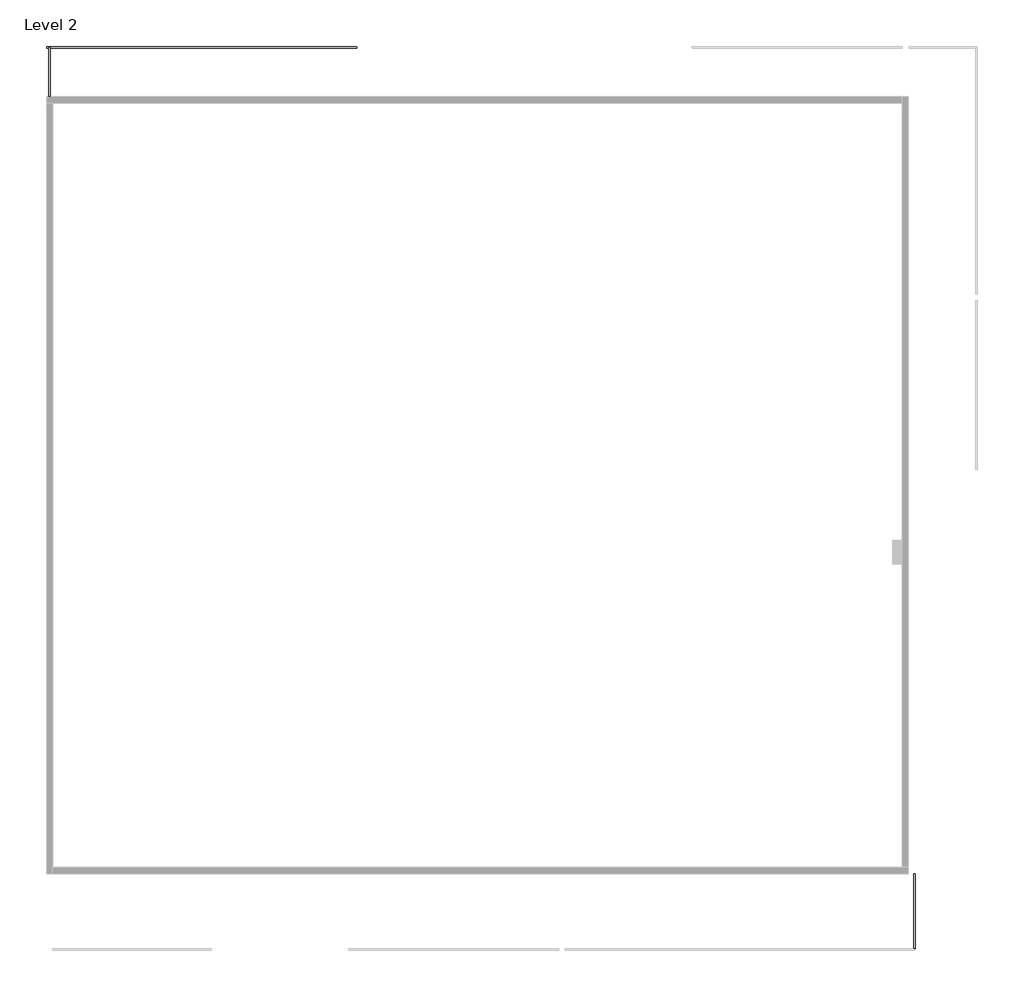
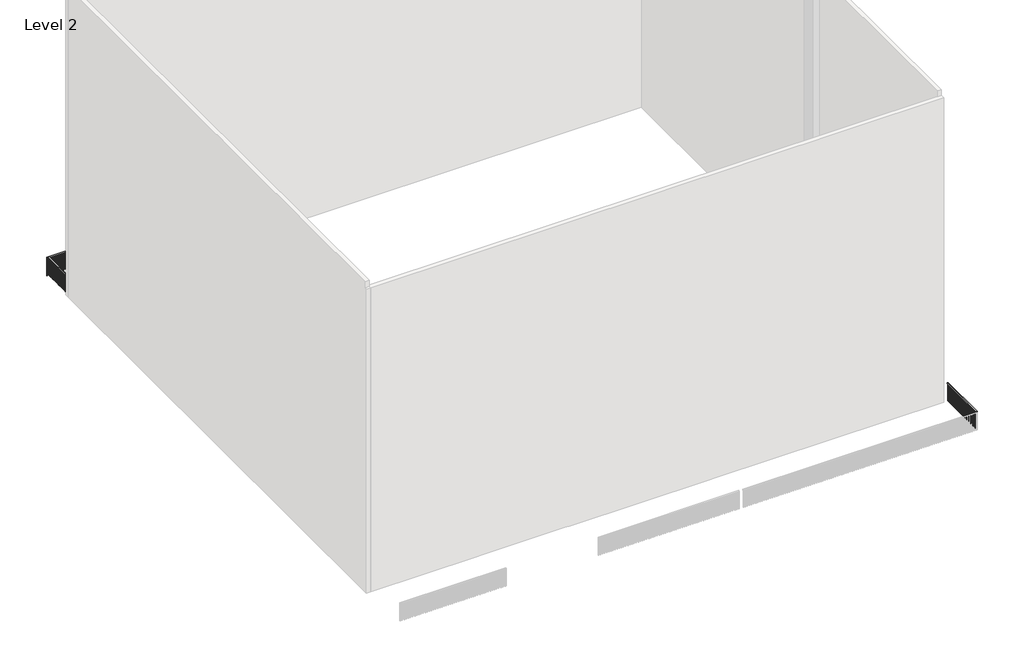
# One storey, part 3 of 5: 3 railings.
"""IFC4 building model written with IfcOpenShell, lengths in millimetres."""

from ifc_helpers import new_model, si_unit, frame, origin, place, context, project, spatial, polyline, outline, extrude, element, save

model = new_model("IFC4")

# Units and contexts
model_context = context("Model", 3, world=origin())
ifc_project = project(units=[si_unit("LENGTHUNIT", "METRE", prefix="MILLI")], contexts=[model_context])

# Site, building, storey
site = spatial("IfcSite", under=ifc_project)
building = spatial("IfcBuilding", under=site)
storey = spatial("IfcBuildingStorey", under=building, Name="Level 2", Elevation=3048.0)

# Railings
placement = place(None, origin())
element("IfcRailing", 1, ObjectType="Handrail - Rectangular", at=placement, inside=storey, context=model_context, shape_type="SweptSolid", body=[
    extrude(outline(polyline([(14335.1361222, -12860.9749501), (14284.3361222, -12860.9749501), (14284.3361222, -10428.1762475), (14335.1361222, -10428.1762475), (14335.1361222, -12860.9749501)])), frame((0.0, 0.0, 3911.6), z_axis=(0.0, 0.0, 1.0), x_axis=(1.0, 0.0, 0.0)), (0.0, 0.0, 1.0), 50.8),
    extrude(outline(polyline([(14319.2611222, -10533.6999501), (14300.2111222, -10533.6999501), (14300.2111222, -10514.6499501), (14319.2611222, -10514.6499501), (14319.2611222, -10533.6999501)])), frame((0.0, 0.0, 3048.0), z_axis=(0.0, 0.0, 1.0), x_axis=(1.0, 0.0, 0.0)), (0.0, 0.0, 1.0), 863.6),
    extrude(outline(polyline([(14319.2611222, -10635.2999501), (14300.2111222, -10635.2999501), (14300.2111222, -10616.2499501), (14319.2611222, -10616.2499501), (14319.2611222, -10635.2999501)])), frame((0.0, 0.0, 3048.0), z_axis=(0.0, 0.0, 1.0), x_axis=(1.0, 0.0, 0.0)), (0.0, 0.0, 1.0), 863.6),
    extrude(outline(polyline([(14319.2611222, -10736.8999501), (14300.2111222, -10736.8999501), (14300.2111222, -10717.8499501), (14319.2611222, -10717.8499501), (14319.2611222, -10736.8999501)])), frame((0.0, 0.0, 3048.0), z_axis=(0.0, 0.0, 1.0), x_axis=(1.0, 0.0, 0.0)), (0.0, 0.0, 1.0), 863.6),
    extrude(outline(polyline([(14319.2611222, -10838.4999501), (14300.2111222, -10838.4999501), (14300.2111222, -10819.4499501), (14319.2611222, -10819.4499501), (14319.2611222, -10838.4999501)])), frame((0.0, 0.0, 3048.0), z_axis=(0.0, 0.0, 1.0), x_axis=(1.0, 0.0, 0.0)), (0.0, 0.0, 1.0), 863.6),
    extrude(outline(polyline([(14319.2611222, -10940.0999501), (14300.2111222, -10940.0999501), (14300.2111222, -10921.0499501), (14319.2611222, -10921.0499501), (14319.2611222, -10940.0999501)])), frame((0.0, 0.0, 3048.0), z_axis=(0.0, 0.0, 1.0), x_axis=(1.0, 0.0, 0.0)), (0.0, 0.0, 1.0), 863.6),
    extrude(outline(polyline([(14319.2611222, -11041.6999501), (14300.2111222, -11041.6999501), (14300.2111222, -11022.6499501), (14319.2611222, -11022.6499501), (14319.2611222, -11041.6999501)])), frame((0.0, 0.0, 3048.0), z_axis=(0.0, 0.0, 1.0), x_axis=(1.0, 0.0, 0.0)), (0.0, 0.0, 1.0), 863.6),
    extrude(outline(polyline([(14319.2611222, -11143.2999501), (14300.2111222, -11143.2999501), (14300.2111222, -11124.2499501), (14319.2611222, -11124.2499501), (14319.2611222, -11143.2999501)])), frame((0.0, 0.0, 3048.0), z_axis=(0.0, 0.0, 1.0), x_axis=(1.0, 0.0, 0.0)), (0.0, 0.0, 1.0), 863.6),
    extrude(outline(polyline([(14319.2611222, -11244.8999501), (14300.2111222, -11244.8999501), (14300.2111222, -11225.8499501), (14319.2611222, -11225.8499501), (14319.2611222, -11244.8999501)])), frame((0.0, 0.0, 3048.0), z_axis=(0.0, 0.0, 1.0), x_axis=(1.0, 0.0, 0.0)), (0.0, 0.0, 1.0), 863.6),
    extrude(outline(polyline([(14319.2611222, -11346.4999501), (14300.2111222, -11346.4999501), (14300.2111222, -11327.4499501), (14319.2611222, -11327.4499501), (14319.2611222, -11346.4999501)])), frame((0.0, 0.0, 3048.0), z_axis=(0.0, 0.0, 1.0), x_axis=(1.0, 0.0, 0.0)), (0.0, 0.0, 1.0), 863.6),
    extrude(outline(polyline([(14319.2611222, -11448.0999501), (14300.2111222, -11448.0999501), (14300.2111222, -11429.0499501), (14319.2611222, -11429.0499501), (14319.2611222, -11448.0999501)])), frame((0.0, 0.0, 3048.0), z_axis=(0.0, 0.0, 1.0), x_axis=(1.0, 0.0, 0.0)), (0.0, 0.0, 1.0), 863.6),
    extrude(outline(polyline([(14319.2611222, -11549.6999501), (14300.2111222, -11549.6999501), (14300.2111222, -11530.6499501), (14319.2611222, -11530.6499501), (14319.2611222, -11549.6999501)])), frame((0.0, 0.0, 3048.0), z_axis=(0.0, 0.0, 1.0), x_axis=(1.0, 0.0, 0.0)), (0.0, 0.0, 1.0), 863.6),
    extrude(outline(polyline([(14319.2611222, -11651.2999501), (14300.2111222, -11651.2999501), (14300.2111222, -11632.2499501), (14319.2611222, -11632.2499501), (14319.2611222, -11651.2999501)])), frame((0.0, 0.0, 3048.0), z_axis=(0.0, 0.0, 1.0), x_axis=(1.0, 0.0, 0.0)), (0.0, 0.0, 1.0), 863.6),
    extrude(outline(polyline([(14319.2611222, -11752.8999501), (14300.2111222, -11752.8999501), (14300.2111222, -11733.8499501), (14319.2611222, -11733.8499501), (14319.2611222, -11752.8999501)])), frame((0.0, 0.0, 3048.0), z_axis=(0.0, 0.0, 1.0), x_axis=(1.0, 0.0, 0.0)), (0.0, 0.0, 1.0), 863.6),
    extrude(outline(polyline([(14319.2611222, -11854.4999501), (14300.2111222, -11854.4999501), (14300.2111222, -11835.4499501), (14319.2611222, -11835.4499501), (14319.2611222, -11854.4999501)])), frame((0.0, 0.0, 3048.0), z_axis=(0.0, 0.0, 1.0), x_axis=(1.0, 0.0, 0.0)), (0.0, 0.0, 1.0), 863.6),
    extrude(outline(polyline([(14319.2611222, -11956.0999501), (14300.2111222, -11956.0999501), (14300.2111222, -11937.0499501), (14319.2611222, -11937.0499501), (14319.2611222, -11956.0999501)])), frame((0.0, 0.0, 3048.0), z_axis=(0.0, 0.0, 1.0), x_axis=(1.0, 0.0, 0.0)), (0.0, 0.0, 1.0), 863.6),
    extrude(outline(polyline([(14319.2611222, -12057.6999501), (14300.2111222, -12057.6999501), (14300.2111222, -12038.6499501), (14319.2611222, -12038.6499501), (14319.2611222, -12057.6999501)])), frame((0.0, 0.0, 3048.0), z_axis=(0.0, 0.0, 1.0), x_axis=(1.0, 0.0, 0.0)), (0.0, 0.0, 1.0), 863.6),
    extrude(outline(polyline([(14319.2611222, -12159.2999501), (14300.2111222, -12159.2999501), (14300.2111222, -12140.2499501), (14319.2611222, -12140.2499501), (14319.2611222, -12159.2999501)])), frame((0.0, 0.0, 3048.0), z_axis=(0.0, 0.0, 1.0), x_axis=(1.0, 0.0, 0.0)), (0.0, 0.0, 1.0), 863.6),
    extrude(outline(polyline([(14319.2611222, -12260.8999501), (14300.2111222, -12260.8999501), (14300.2111222, -12241.8499501), (14319.2611222, -12241.8499501), (14319.2611222, -12260.8999501)])), frame((0.0, 0.0, 3048.0), z_axis=(0.0, 0.0, 1.0), x_axis=(1.0, 0.0, 0.0)), (0.0, 0.0, 1.0), 863.6),
    extrude(outline(polyline([(14319.2611222, -12362.4999501), (14300.2111222, -12362.4999501), (14300.2111222, -12343.4499501), (14319.2611222, -12343.4499501), (14319.2611222, -12362.4999501)])), frame((0.0, 0.0, 3048.0), z_axis=(0.0, 0.0, 1.0), x_axis=(1.0, 0.0, 0.0)), (0.0, 0.0, 1.0), 863.6),
    extrude(outline(polyline([(14319.2611222, -12464.0999501), (14300.2111222, -12464.0999501), (14300.2111222, -12445.0499501), (14319.2611222, -12445.0499501), (14319.2611222, -12464.0999501)])), frame((0.0, 0.0, 3048.0), z_axis=(0.0, 0.0, 1.0), x_axis=(1.0, 0.0, 0.0)), (0.0, 0.0, 1.0), 863.6),
    extrude(outline(polyline([(14319.2611222, -12565.6999501), (14300.2111222, -12565.6999501), (14300.2111222, -12546.6499501), (14319.2611222, -12546.6499501), (14319.2611222, -12565.6999501)])), frame((0.0, 0.0, 3048.0), z_axis=(0.0, 0.0, 1.0), x_axis=(1.0, 0.0, 0.0)), (0.0, 0.0, 1.0), 863.6),
    extrude(outline(polyline([(14319.2611222, -12667.2999501), (14300.2111222, -12667.2999501), (14300.2111222, -12648.2499501), (14319.2611222, -12648.2499501), (14319.2611222, -12667.2999501)])), frame((0.0, 0.0, 3048.0), z_axis=(0.0, 0.0, 1.0), x_axis=(1.0, 0.0, 0.0)), (0.0, 0.0, 1.0), 863.6),
    extrude(outline(polyline([(14319.2611222, -12768.8999501), (14300.2111222, -12768.8999501), (14300.2111222, -12749.8499501), (14319.2611222, -12749.8499501), (14319.2611222, -12768.8999501)])), frame((0.0, 0.0, 3048.0), z_axis=(0.0, 0.0, 1.0), x_axis=(1.0, 0.0, 0.0)), (0.0, 0.0, 1.0), 863.6),
    extrude(outline(polyline([(14319.2611222, -10447.2262475), (14300.2111222, -10447.2262475), (14300.2111222, -10428.1762475), (14319.2611222, -10428.1762475), (14319.2611222, -10447.2262475)])), frame((0.0, 0.0, 3048.0), z_axis=(0.0, 0.0, 1.0), x_axis=(1.0, 0.0, 0.0)), (0.0, 0.0, 1.0), 863.6),
    extrude(outline(polyline([(14319.2611222, -12860.9749501), (14300.2111222, -12860.9749501), (14300.2111222, -12841.9249501), (14319.2611222, -12841.9249501), (14319.2611222, -12860.9749501)])), frame((0.0, 0.0, 3048.0), z_axis=(0.0, 0.0, 1.0), x_axis=(1.0, 0.0, 0.0)), (0.0, 0.0, 1.0), 863.6),
])
element("IfcRailing", 2, ObjectType="Handrail - Rectangular", at=placement, inside=storey, context=model_context, shape_type="SweptSolid", body=[
    extrude(outline(polyline([(-3775.0638778, 16399.8250499), (-3775.0638778, 16349.0250499), (-13833.4638778, 16349.0250499), (-13833.4638778, 16399.8250499), (-3775.0638778, 16399.8250499)])), frame((0.0, 0.0, 3911.6), z_axis=(0.0, 0.0, 1.0), x_axis=(1.0, 0.0, 0.0)), (0.0, 0.0, 1.0), 50.8),
    extrude(outline(polyline([(-13722.3388778, 16383.9500499), (-13722.3388778, 16364.9000499), (-13741.3888778, 16364.9000499), (-13741.3888778, 16383.9500499), (-13722.3388778, 16383.9500499)])), frame((0.0, 0.0, 3048.0), z_axis=(0.0, 0.0, 1.0), x_axis=(1.0, 0.0, 0.0)), (0.0, 0.0, 1.0), 863.6),
    extrude(outline(polyline([(-13620.7388778, 16383.9500499), (-13620.7388778, 16364.9000499), (-13639.7888778, 16364.9000499), (-13639.7888778, 16383.9500499), (-13620.7388778, 16383.9500499)])), frame((0.0, 0.0, 3048.0), z_axis=(0.0, 0.0, 1.0), x_axis=(1.0, 0.0, 0.0)), (0.0, 0.0, 1.0), 863.6),
    extrude(outline(polyline([(-13519.1388778, 16383.9500499), (-13519.1388778, 16364.9000499), (-13538.1888778, 16364.9000499), (-13538.1888778, 16383.9500499), (-13519.1388778, 16383.9500499)])), frame((0.0, 0.0, 3048.0), z_axis=(0.0, 0.0, 1.0), x_axis=(1.0, 0.0, 0.0)), (0.0, 0.0, 1.0), 863.6),
    extrude(outline(polyline([(-13417.5388778, 16383.9500499), (-13417.5388778, 16364.9000499), (-13436.5888778, 16364.9000499), (-13436.5888778, 16383.9500499), (-13417.5388778, 16383.9500499)])), frame((0.0, 0.0, 3048.0), z_axis=(0.0, 0.0, 1.0), x_axis=(1.0, 0.0, 0.0)), (0.0, 0.0, 1.0), 863.6),
    extrude(outline(polyline([(-13315.9388778, 16383.9500499), (-13315.9388778, 16364.9000499), (-13334.9888778, 16364.9000499), (-13334.9888778, 16383.9500499), (-13315.9388778, 16383.9500499)])), frame((0.0, 0.0, 3048.0), z_axis=(0.0, 0.0, 1.0), x_axis=(1.0, 0.0, 0.0)), (0.0, 0.0, 1.0), 863.6),
    extrude(outline(polyline([(-13214.3388778, 16383.9500499), (-13214.3388778, 16364.9000499), (-13233.3888778, 16364.9000499), (-13233.3888778, 16383.9500499), (-13214.3388778, 16383.9500499)])), frame((0.0, 0.0, 3048.0), z_axis=(0.0, 0.0, 1.0), x_axis=(1.0, 0.0, 0.0)), (0.0, 0.0, 1.0), 863.6),
    extrude(outline(polyline([(-13112.7388778, 16383.9500499), (-13112.7388778, 16364.9000499), (-13131.7888778, 16364.9000499), (-13131.7888778, 16383.9500499), (-13112.7388778, 16383.9500499)])), frame((0.0, 0.0, 3048.0), z_axis=(0.0, 0.0, 1.0), x_axis=(1.0, 0.0, 0.0)), (0.0, 0.0, 1.0), 863.6),
    extrude(outline(polyline([(-13011.1388778, 16383.9500499), (-13011.1388778, 16364.9000499), (-13030.1888778, 16364.9000499), (-13030.1888778, 16383.9500499), (-13011.1388778, 16383.9500499)])), frame((0.0, 0.0, 3048.0), z_axis=(0.0, 0.0, 1.0), x_axis=(1.0, 0.0, 0.0)), (0.0, 0.0, 1.0), 863.6),
    extrude(outline(polyline([(-12909.5388778, 16383.9500499), (-12909.5388778, 16364.9000499), (-12928.5888778, 16364.9000499), (-12928.5888778, 16383.9500499), (-12909.5388778, 16383.9500499)])), frame((0.0, 0.0, 3048.0), z_axis=(0.0, 0.0, 1.0), x_axis=(1.0, 0.0, 0.0)), (0.0, 0.0, 1.0), 863.6),
    extrude(outline(polyline([(-12807.9388778, 16383.9500499), (-12807.9388778, 16364.9000499), (-12826.9888778, 16364.9000499), (-12826.9888778, 16383.9500499), (-12807.9388778, 16383.9500499)])), frame((0.0, 0.0, 3048.0), z_axis=(0.0, 0.0, 1.0), x_axis=(1.0, 0.0, 0.0)), (0.0, 0.0, 1.0), 863.6),
    extrude(outline(polyline([(-12706.3388778, 16383.9500499), (-12706.3388778, 16364.9000499), (-12725.3888778, 16364.9000499), (-12725.3888778, 16383.9500499), (-12706.3388778, 16383.9500499)])), frame((0.0, 0.0, 3048.0), z_axis=(0.0, 0.0, 1.0), x_axis=(1.0, 0.0, 0.0)), (0.0, 0.0, 1.0), 863.6),
    extrude(outline(polyline([(-12604.7388778, 16383.9500499), (-12604.7388778, 16364.9000499), (-12623.7888778, 16364.9000499), (-12623.7888778, 16383.9500499), (-12604.7388778, 16383.9500499)])), frame((0.0, 0.0, 3048.0), z_axis=(0.0, 0.0, 1.0), x_axis=(1.0, 0.0, 0.0)), (0.0, 0.0, 1.0), 863.6),
    extrude(outline(polyline([(-12503.1388778, 16383.9500499), (-12503.1388778, 16364.9000499), (-12522.1888778, 16364.9000499), (-12522.1888778, 16383.9500499), (-12503.1388778, 16383.9500499)])), frame((0.0, 0.0, 3048.0), z_axis=(0.0, 0.0, 1.0), x_axis=(1.0, 0.0, 0.0)), (0.0, 0.0, 1.0), 863.6),
    extrude(outline(polyline([(-12401.5388778, 16383.9500499), (-12401.5388778, 16364.9000499), (-12420.5888778, 16364.9000499), (-12420.5888778, 16383.9500499), (-12401.5388778, 16383.9500499)])), frame((0.0, 0.0, 3048.0), z_axis=(0.0, 0.0, 1.0), x_axis=(1.0, 0.0, 0.0)), (0.0, 0.0, 1.0), 863.6),
    extrude(outline(polyline([(-12299.9388778, 16383.9500499), (-12299.9388778, 16364.9000499), (-12318.9888778, 16364.9000499), (-12318.9888778, 16383.9500499), (-12299.9388778, 16383.9500499)])), frame((0.0, 0.0, 3048.0), z_axis=(0.0, 0.0, 1.0), x_axis=(1.0, 0.0, 0.0)), (0.0, 0.0, 1.0), 863.6),
    extrude(outline(polyline([(-12198.3388778, 16383.9500499), (-12198.3388778, 16364.9000499), (-12217.3888778, 16364.9000499), (-12217.3888778, 16383.9500499), (-12198.3388778, 16383.9500499)])), frame((0.0, 0.0, 3048.0), z_axis=(0.0, 0.0, 1.0), x_axis=(1.0, 0.0, 0.0)), (0.0, 0.0, 1.0), 863.6),
    extrude(outline(polyline([(-12096.7388778, 16383.9500499), (-12096.7388778, 16364.9000499), (-12115.7888778, 16364.9000499), (-12115.7888778, 16383.9500499), (-12096.7388778, 16383.9500499)])), frame((0.0, 0.0, 3048.0), z_axis=(0.0, 0.0, 1.0), x_axis=(1.0, 0.0, 0.0)), (0.0, 0.0, 1.0), 863.6),
    extrude(outline(polyline([(-11995.1388778, 16383.9500499), (-11995.1388778, 16364.9000499), (-12014.1888778, 16364.9000499), (-12014.1888778, 16383.9500499), (-11995.1388778, 16383.9500499)])), frame((0.0, 0.0, 3048.0), z_axis=(0.0, 0.0, 1.0), x_axis=(1.0, 0.0, 0.0)), (0.0, 0.0, 1.0), 863.6),
    extrude(outline(polyline([(-11893.5388778, 16383.9500499), (-11893.5388778, 16364.9000499), (-11912.5888778, 16364.9000499), (-11912.5888778, 16383.9500499), (-11893.5388778, 16383.9500499)])), frame((0.0, 0.0, 3048.0), z_axis=(0.0, 0.0, 1.0), x_axis=(1.0, 0.0, 0.0)), (0.0, 0.0, 1.0), 863.6),
    extrude(outline(polyline([(-11791.9388778, 16383.9500499), (-11791.9388778, 16364.9000499), (-11810.9888778, 16364.9000499), (-11810.9888778, 16383.9500499), (-11791.9388778, 16383.9500499)])), frame((0.0, 0.0, 3048.0), z_axis=(0.0, 0.0, 1.0), x_axis=(1.0, 0.0, 0.0)), (0.0, 0.0, 1.0), 863.6),
    extrude(outline(polyline([(-11690.3388778, 16383.9500499), (-11690.3388778, 16364.9000499), (-11709.3888778, 16364.9000499), (-11709.3888778, 16383.9500499), (-11690.3388778, 16383.9500499)])), frame((0.0, 0.0, 3048.0), z_axis=(0.0, 0.0, 1.0), x_axis=(1.0, 0.0, 0.0)), (0.0, 0.0, 1.0), 863.6),
    extrude(outline(polyline([(-11588.7388778, 16383.9500499), (-11588.7388778, 16364.9000499), (-11607.7888778, 16364.9000499), (-11607.7888778, 16383.9500499), (-11588.7388778, 16383.9500499)])), frame((0.0, 0.0, 3048.0), z_axis=(0.0, 0.0, 1.0), x_axis=(1.0, 0.0, 0.0)), (0.0, 0.0, 1.0), 863.6),
    extrude(outline(polyline([(-11487.1388778, 16383.9500499), (-11487.1388778, 16364.9000499), (-11506.1888778, 16364.9000499), (-11506.1888778, 16383.9500499), (-11487.1388778, 16383.9500499)])), frame((0.0, 0.0, 3048.0), z_axis=(0.0, 0.0, 1.0), x_axis=(1.0, 0.0, 0.0)), (0.0, 0.0, 1.0), 863.6),
    extrude(outline(polyline([(-11385.5388778, 16383.9500499), (-11385.5388778, 16364.9000499), (-11404.5888778, 16364.9000499), (-11404.5888778, 16383.9500499), (-11385.5388778, 16383.9500499)])), frame((0.0, 0.0, 3048.0), z_axis=(0.0, 0.0, 1.0), x_axis=(1.0, 0.0, 0.0)), (0.0, 0.0, 1.0), 863.6),
    extrude(outline(polyline([(-11283.9388778, 16383.9500499), (-11283.9388778, 16364.9000499), (-11302.9888778, 16364.9000499), (-11302.9888778, 16383.9500499), (-11283.9388778, 16383.9500499)])), frame((0.0, 0.0, 3048.0), z_axis=(0.0, 0.0, 1.0), x_axis=(1.0, 0.0, 0.0)), (0.0, 0.0, 1.0), 863.6),
    extrude(outline(polyline([(-11182.3388778, 16383.9500499), (-11182.3388778, 16364.9000499), (-11201.3888778, 16364.9000499), (-11201.3888778, 16383.9500499), (-11182.3388778, 16383.9500499)])), frame((0.0, 0.0, 3048.0), z_axis=(0.0, 0.0, 1.0), x_axis=(1.0, 0.0, 0.0)), (0.0, 0.0, 1.0), 863.6),
    extrude(outline(polyline([(-11080.7388778, 16383.9500499), (-11080.7388778, 16364.9000499), (-11099.7888778, 16364.9000499), (-11099.7888778, 16383.9500499), (-11080.7388778, 16383.9500499)])), frame((0.0, 0.0, 3048.0), z_axis=(0.0, 0.0, 1.0), x_axis=(1.0, 0.0, 0.0)), (0.0, 0.0, 1.0), 863.6),
    extrude(outline(polyline([(-10979.1388778, 16383.9500499), (-10979.1388778, 16364.9000499), (-10998.1888778, 16364.9000499), (-10998.1888778, 16383.9500499), (-10979.1388778, 16383.9500499)])), frame((0.0, 0.0, 3048.0), z_axis=(0.0, 0.0, 1.0), x_axis=(1.0, 0.0, 0.0)), (0.0, 0.0, 1.0), 863.6),
    extrude(outline(polyline([(-10877.5388778, 16383.9500499), (-10877.5388778, 16364.9000499), (-10896.5888778, 16364.9000499), (-10896.5888778, 16383.9500499), (-10877.5388778, 16383.9500499)])), frame((0.0, 0.0, 3048.0), z_axis=(0.0, 0.0, 1.0), x_axis=(1.0, 0.0, 0.0)), (0.0, 0.0, 1.0), 863.6),
    extrude(outline(polyline([(-10775.9388778, 16383.9500499), (-10775.9388778, 16364.9000499), (-10794.9888778, 16364.9000499), (-10794.9888778, 16383.9500499), (-10775.9388778, 16383.9500499)])), frame((0.0, 0.0, 3048.0), z_axis=(0.0, 0.0, 1.0), x_axis=(1.0, 0.0, 0.0)), (0.0, 0.0, 1.0), 863.6),
    extrude(outline(polyline([(-10674.3388778, 16383.9500499), (-10674.3388778, 16364.9000499), (-10693.3888778, 16364.9000499), (-10693.3888778, 16383.9500499), (-10674.3388778, 16383.9500499)])), frame((0.0, 0.0, 3048.0), z_axis=(0.0, 0.0, 1.0), x_axis=(1.0, 0.0, 0.0)), (0.0, 0.0, 1.0), 863.6),
    extrude(outline(polyline([(-10572.7388778, 16383.9500499), (-10572.7388778, 16364.9000499), (-10591.7888778, 16364.9000499), (-10591.7888778, 16383.9500499), (-10572.7388778, 16383.9500499)])), frame((0.0, 0.0, 3048.0), z_axis=(0.0, 0.0, 1.0), x_axis=(1.0, 0.0, 0.0)), (0.0, 0.0, 1.0), 863.6),
    extrude(outline(polyline([(-10471.1388778, 16383.9500499), (-10471.1388778, 16364.9000499), (-10490.1888778, 16364.9000499), (-10490.1888778, 16383.9500499), (-10471.1388778, 16383.9500499)])), frame((0.0, 0.0, 3048.0), z_axis=(0.0, 0.0, 1.0), x_axis=(1.0, 0.0, 0.0)), (0.0, 0.0, 1.0), 863.6),
    extrude(outline(polyline([(-10369.5388778, 16383.9500499), (-10369.5388778, 16364.9000499), (-10388.5888778, 16364.9000499), (-10388.5888778, 16383.9500499), (-10369.5388778, 16383.9500499)])), frame((0.0, 0.0, 3048.0), z_axis=(0.0, 0.0, 1.0), x_axis=(1.0, 0.0, 0.0)), (0.0, 0.0, 1.0), 863.6),
    extrude(outline(polyline([(-10267.9388778, 16383.9500499), (-10267.9388778, 16364.9000499), (-10286.9888778, 16364.9000499), (-10286.9888778, 16383.9500499), (-10267.9388778, 16383.9500499)])), frame((0.0, 0.0, 3048.0), z_axis=(0.0, 0.0, 1.0), x_axis=(1.0, 0.0, 0.0)), (0.0, 0.0, 1.0), 863.6),
    extrude(outline(polyline([(-10166.3388778, 16383.9500499), (-10166.3388778, 16364.9000499), (-10185.3888778, 16364.9000499), (-10185.3888778, 16383.9500499), (-10166.3388778, 16383.9500499)])), frame((0.0, 0.0, 3048.0), z_axis=(0.0, 0.0, 1.0), x_axis=(1.0, 0.0, 0.0)), (0.0, 0.0, 1.0), 863.6),
    extrude(outline(polyline([(-10064.7388778, 16383.9500499), (-10064.7388778, 16364.9000499), (-10083.7888778, 16364.9000499), (-10083.7888778, 16383.9500499), (-10064.7388778, 16383.9500499)])), frame((0.0, 0.0, 3048.0), z_axis=(0.0, 0.0, 1.0), x_axis=(1.0, 0.0, 0.0)), (0.0, 0.0, 1.0), 863.6),
    extrude(outline(polyline([(-9963.1388778, 16383.9500499), (-9963.1388778, 16364.9000499), (-9982.1888778, 16364.9000499), (-9982.1888778, 16383.9500499), (-9963.1388778, 16383.9500499)])), frame((0.0, 0.0, 3048.0), z_axis=(0.0, 0.0, 1.0), x_axis=(1.0, 0.0, 0.0)), (0.0, 0.0, 1.0), 863.6),
    extrude(outline(polyline([(-9861.5388778, 16383.9500499), (-9861.5388778, 16364.9000499), (-9880.5888778, 16364.9000499), (-9880.5888778, 16383.9500499), (-9861.5388778, 16383.9500499)])), frame((0.0, 0.0, 3048.0), z_axis=(0.0, 0.0, 1.0), x_axis=(1.0, 0.0, 0.0)), (0.0, 0.0, 1.0), 863.6),
    extrude(outline(polyline([(-9759.9388778, 16383.9500499), (-9759.9388778, 16364.9000499), (-9778.9888778, 16364.9000499), (-9778.9888778, 16383.9500499), (-9759.9388778, 16383.9500499)])), frame((0.0, 0.0, 3048.0), z_axis=(0.0, 0.0, 1.0), x_axis=(1.0, 0.0, 0.0)), (0.0, 0.0, 1.0), 863.6),
    extrude(outline(polyline([(-9658.3388778, 16383.9500499), (-9658.3388778, 16364.9000499), (-9677.3888778, 16364.9000499), (-9677.3888778, 16383.9500499), (-9658.3388778, 16383.9500499)])), frame((0.0, 0.0, 3048.0), z_axis=(0.0, 0.0, 1.0), x_axis=(1.0, 0.0, 0.0)), (0.0, 0.0, 1.0), 863.6),
    extrude(outline(polyline([(-9556.7388778, 16383.9500499), (-9556.7388778, 16364.9000499), (-9575.7888778, 16364.9000499), (-9575.7888778, 16383.9500499), (-9556.7388778, 16383.9500499)])), frame((0.0, 0.0, 3048.0), z_axis=(0.0, 0.0, 1.0), x_axis=(1.0, 0.0, 0.0)), (0.0, 0.0, 1.0), 863.6),
    extrude(outline(polyline([(-9455.1388778, 16383.9500499), (-9455.1388778, 16364.9000499), (-9474.1888778, 16364.9000499), (-9474.1888778, 16383.9500499), (-9455.1388778, 16383.9500499)])), frame((0.0, 0.0, 3048.0), z_axis=(0.0, 0.0, 1.0), x_axis=(1.0, 0.0, 0.0)), (0.0, 0.0, 1.0), 863.6),
    extrude(outline(polyline([(-9353.5388778, 16383.9500499), (-9353.5388778, 16364.9000499), (-9372.5888778, 16364.9000499), (-9372.5888778, 16383.9500499), (-9353.5388778, 16383.9500499)])), frame((0.0, 0.0, 3048.0), z_axis=(0.0, 0.0, 1.0), x_axis=(1.0, 0.0, 0.0)), (0.0, 0.0, 1.0), 863.6),
    extrude(outline(polyline([(-9251.9388778, 16383.9500499), (-9251.9388778, 16364.9000499), (-9270.9888778, 16364.9000499), (-9270.9888778, 16383.9500499), (-9251.9388778, 16383.9500499)])), frame((0.0, 0.0, 3048.0), z_axis=(0.0, 0.0, 1.0), x_axis=(1.0, 0.0, 0.0)), (0.0, 0.0, 1.0), 863.6),
    extrude(outline(polyline([(-9150.3388778, 16383.9500499), (-9150.3388778, 16364.9000499), (-9169.3888778, 16364.9000499), (-9169.3888778, 16383.9500499), (-9150.3388778, 16383.9500499)])), frame((0.0, 0.0, 3048.0), z_axis=(0.0, 0.0, 1.0), x_axis=(1.0, 0.0, 0.0)), (0.0, 0.0, 1.0), 863.6),
    extrude(outline(polyline([(-9048.7388778, 16383.9500499), (-9048.7388778, 16364.9000499), (-9067.7888778, 16364.9000499), (-9067.7888778, 16383.9500499), (-9048.7388778, 16383.9500499)])), frame((0.0, 0.0, 3048.0), z_axis=(0.0, 0.0, 1.0), x_axis=(1.0, 0.0, 0.0)), (0.0, 0.0, 1.0), 863.6),
    extrude(outline(polyline([(-8947.1388778, 16383.9500499), (-8947.1388778, 16364.9000499), (-8966.1888778, 16364.9000499), (-8966.1888778, 16383.9500499), (-8947.1388778, 16383.9500499)])), frame((0.0, 0.0, 3048.0), z_axis=(0.0, 0.0, 1.0), x_axis=(1.0, 0.0, 0.0)), (0.0, 0.0, 1.0), 863.6),
    extrude(outline(polyline([(-8845.5388778, 16383.9500499), (-8845.5388778, 16364.9000499), (-8864.5888778, 16364.9000499), (-8864.5888778, 16383.9500499), (-8845.5388778, 16383.9500499)])), frame((0.0, 0.0, 3048.0), z_axis=(0.0, 0.0, 1.0), x_axis=(1.0, 0.0, 0.0)), (0.0, 0.0, 1.0), 863.6),
    extrude(outline(polyline([(-8743.9388778, 16383.9500499), (-8743.9388778, 16364.9000499), (-8762.9888778, 16364.9000499), (-8762.9888778, 16383.9500499), (-8743.9388778, 16383.9500499)])), frame((0.0, 0.0, 3048.0), z_axis=(0.0, 0.0, 1.0), x_axis=(1.0, 0.0, 0.0)), (0.0, 0.0, 1.0), 863.6),
    extrude(outline(polyline([(-8642.3388778, 16383.9500499), (-8642.3388778, 16364.9000499), (-8661.3888778, 16364.9000499), (-8661.3888778, 16383.9500499), (-8642.3388778, 16383.9500499)])), frame((0.0, 0.0, 3048.0), z_axis=(0.0, 0.0, 1.0), x_axis=(1.0, 0.0, 0.0)), (0.0, 0.0, 1.0), 863.6),
    extrude(outline(polyline([(-8540.7388778, 16383.9500499), (-8540.7388778, 16364.9000499), (-8559.7888778, 16364.9000499), (-8559.7888778, 16383.9500499), (-8540.7388778, 16383.9500499)])), frame((0.0, 0.0, 3048.0), z_axis=(0.0, 0.0, 1.0), x_axis=(1.0, 0.0, 0.0)), (0.0, 0.0, 1.0), 863.6),
    extrude(outline(polyline([(-8439.1388778, 16383.9500499), (-8439.1388778, 16364.9000499), (-8458.1888778, 16364.9000499), (-8458.1888778, 16383.9500499), (-8439.1388778, 16383.9500499)])), frame((0.0, 0.0, 3048.0), z_axis=(0.0, 0.0, 1.0), x_axis=(1.0, 0.0, 0.0)), (0.0, 0.0, 1.0), 863.6),
    extrude(outline(polyline([(-8337.5388778, 16383.9500499), (-8337.5388778, 16364.9000499), (-8356.5888778, 16364.9000499), (-8356.5888778, 16383.9500499), (-8337.5388778, 16383.9500499)])), frame((0.0, 0.0, 3048.0), z_axis=(0.0, 0.0, 1.0), x_axis=(1.0, 0.0, 0.0)), (0.0, 0.0, 1.0), 863.6),
    extrude(outline(polyline([(-8235.9388778, 16383.9500499), (-8235.9388778, 16364.9000499), (-8254.9888778, 16364.9000499), (-8254.9888778, 16383.9500499), (-8235.9388778, 16383.9500499)])), frame((0.0, 0.0, 3048.0), z_axis=(0.0, 0.0, 1.0), x_axis=(1.0, 0.0, 0.0)), (0.0, 0.0, 1.0), 863.6),
    extrude(outline(polyline([(-8134.3388778, 16383.9500499), (-8134.3388778, 16364.9000499), (-8153.3888778, 16364.9000499), (-8153.3888778, 16383.9500499), (-8134.3388778, 16383.9500499)])), frame((0.0, 0.0, 3048.0), z_axis=(0.0, 0.0, 1.0), x_axis=(1.0, 0.0, 0.0)), (0.0, 0.0, 1.0), 863.6),
    extrude(outline(polyline([(-8032.7388778, 16383.9500499), (-8032.7388778, 16364.9000499), (-8051.7888778, 16364.9000499), (-8051.7888778, 16383.9500499), (-8032.7388778, 16383.9500499)])), frame((0.0, 0.0, 3048.0), z_axis=(0.0, 0.0, 1.0), x_axis=(1.0, 0.0, 0.0)), (0.0, 0.0, 1.0), 863.6),
    extrude(outline(polyline([(-7931.1388778, 16383.9500499), (-7931.1388778, 16364.9000499), (-7950.1888778, 16364.9000499), (-7950.1888778, 16383.9500499), (-7931.1388778, 16383.9500499)])), frame((0.0, 0.0, 3048.0), z_axis=(0.0, 0.0, 1.0), x_axis=(1.0, 0.0, 0.0)), (0.0, 0.0, 1.0), 863.6),
    extrude(outline(polyline([(-7829.5388778, 16383.9500499), (-7829.5388778, 16364.9000499), (-7848.5888778, 16364.9000499), (-7848.5888778, 16383.9500499), (-7829.5388778, 16383.9500499)])), frame((0.0, 0.0, 3048.0), z_axis=(0.0, 0.0, 1.0), x_axis=(1.0, 0.0, 0.0)), (0.0, 0.0, 1.0), 863.6),
    extrude(outline(polyline([(-7727.9388778, 16383.9500499), (-7727.9388778, 16364.9000499), (-7746.9888778, 16364.9000499), (-7746.9888778, 16383.9500499), (-7727.9388778, 16383.9500499)])), frame((0.0, 0.0, 3048.0), z_axis=(0.0, 0.0, 1.0), x_axis=(1.0, 0.0, 0.0)), (0.0, 0.0, 1.0), 863.6),
    extrude(outline(polyline([(-7626.3388778, 16383.9500499), (-7626.3388778, 16364.9000499), (-7645.3888778, 16364.9000499), (-7645.3888778, 16383.9500499), (-7626.3388778, 16383.9500499)])), frame((0.0, 0.0, 3048.0), z_axis=(0.0, 0.0, 1.0), x_axis=(1.0, 0.0, 0.0)), (0.0, 0.0, 1.0), 863.6),
    extrude(outline(polyline([(-7524.7388778, 16383.9500499), (-7524.7388778, 16364.9000499), (-7543.7888778, 16364.9000499), (-7543.7888778, 16383.9500499), (-7524.7388778, 16383.9500499)])), frame((0.0, 0.0, 3048.0), z_axis=(0.0, 0.0, 1.0), x_axis=(1.0, 0.0, 0.0)), (0.0, 0.0, 1.0), 863.6),
    extrude(outline(polyline([(-7423.1388778, 16383.9500499), (-7423.1388778, 16364.9000499), (-7442.1888778, 16364.9000499), (-7442.1888778, 16383.9500499), (-7423.1388778, 16383.9500499)])), frame((0.0, 0.0, 3048.0), z_axis=(0.0, 0.0, 1.0), x_axis=(1.0, 0.0, 0.0)), (0.0, 0.0, 1.0), 863.6),
    extrude(outline(polyline([(-7321.5388778, 16383.9500499), (-7321.5388778, 16364.9000499), (-7340.5888778, 16364.9000499), (-7340.5888778, 16383.9500499), (-7321.5388778, 16383.9500499)])), frame((0.0, 0.0, 3048.0), z_axis=(0.0, 0.0, 1.0), x_axis=(1.0, 0.0, 0.0)), (0.0, 0.0, 1.0), 863.6),
    extrude(outline(polyline([(-7219.9388778, 16383.9500499), (-7219.9388778, 16364.9000499), (-7238.9888778, 16364.9000499), (-7238.9888778, 16383.9500499), (-7219.9388778, 16383.9500499)])), frame((0.0, 0.0, 3048.0), z_axis=(0.0, 0.0, 1.0), x_axis=(1.0, 0.0, 0.0)), (0.0, 0.0, 1.0), 863.6),
    extrude(outline(polyline([(-7118.3388778, 16383.9500499), (-7118.3388778, 16364.9000499), (-7137.3888778, 16364.9000499), (-7137.3888778, 16383.9500499), (-7118.3388778, 16383.9500499)])), frame((0.0, 0.0, 3048.0), z_axis=(0.0, 0.0, 1.0), x_axis=(1.0, 0.0, 0.0)), (0.0, 0.0, 1.0), 863.6),
    extrude(outline(polyline([(-7016.7388778, 16383.9500499), (-7016.7388778, 16364.9000499), (-7035.7888778, 16364.9000499), (-7035.7888778, 16383.9500499), (-7016.7388778, 16383.9500499)])), frame((0.0, 0.0, 3048.0), z_axis=(0.0, 0.0, 1.0), x_axis=(1.0, 0.0, 0.0)), (0.0, 0.0, 1.0), 863.6),
    extrude(outline(polyline([(-6915.1388778, 16383.9500499), (-6915.1388778, 16364.9000499), (-6934.1888778, 16364.9000499), (-6934.1888778, 16383.9500499), (-6915.1388778, 16383.9500499)])), frame((0.0, 0.0, 3048.0), z_axis=(0.0, 0.0, 1.0), x_axis=(1.0, 0.0, 0.0)), (0.0, 0.0, 1.0), 863.6),
    extrude(outline(polyline([(-6813.5388778, 16383.9500499), (-6813.5388778, 16364.9000499), (-6832.5888778, 16364.9000499), (-6832.5888778, 16383.9500499), (-6813.5388778, 16383.9500499)])), frame((0.0, 0.0, 3048.0), z_axis=(0.0, 0.0, 1.0), x_axis=(1.0, 0.0, 0.0)), (0.0, 0.0, 1.0), 863.6),
    extrude(outline(polyline([(-6711.9388778, 16383.9500499), (-6711.9388778, 16364.9000499), (-6730.9888778, 16364.9000499), (-6730.9888778, 16383.9500499), (-6711.9388778, 16383.9500499)])), frame((0.0, 0.0, 3048.0), z_axis=(0.0, 0.0, 1.0), x_axis=(1.0, 0.0, 0.0)), (0.0, 0.0, 1.0), 863.6),
    extrude(outline(polyline([(-6610.3388778, 16383.9500499), (-6610.3388778, 16364.9000499), (-6629.3888778, 16364.9000499), (-6629.3888778, 16383.9500499), (-6610.3388778, 16383.9500499)])), frame((0.0, 0.0, 3048.0), z_axis=(0.0, 0.0, 1.0), x_axis=(1.0, 0.0, 0.0)), (0.0, 0.0, 1.0), 863.6),
    extrude(outline(polyline([(-6508.7388778, 16383.9500499), (-6508.7388778, 16364.9000499), (-6527.7888778, 16364.9000499), (-6527.7888778, 16383.9500499), (-6508.7388778, 16383.9500499)])), frame((0.0, 0.0, 3048.0), z_axis=(0.0, 0.0, 1.0), x_axis=(1.0, 0.0, 0.0)), (0.0, 0.0, 1.0), 863.6),
    extrude(outline(polyline([(-6407.1388778, 16383.9500499), (-6407.1388778, 16364.9000499), (-6426.1888778, 16364.9000499), (-6426.1888778, 16383.9500499), (-6407.1388778, 16383.9500499)])), frame((0.0, 0.0, 3048.0), z_axis=(0.0, 0.0, 1.0), x_axis=(1.0, 0.0, 0.0)), (0.0, 0.0, 1.0), 863.6),
    extrude(outline(polyline([(-6305.5388778, 16383.9500499), (-6305.5388778, 16364.9000499), (-6324.5888778, 16364.9000499), (-6324.5888778, 16383.9500499), (-6305.5388778, 16383.9500499)])), frame((0.0, 0.0, 3048.0), z_axis=(0.0, 0.0, 1.0), x_axis=(1.0, 0.0, 0.0)), (0.0, 0.0, 1.0), 863.6),
    extrude(outline(polyline([(-6203.9388778, 16383.9500499), (-6203.9388778, 16364.9000499), (-6222.9888778, 16364.9000499), (-6222.9888778, 16383.9500499), (-6203.9388778, 16383.9500499)])), frame((0.0, 0.0, 3048.0), z_axis=(0.0, 0.0, 1.0), x_axis=(1.0, 0.0, 0.0)), (0.0, 0.0, 1.0), 863.6),
    extrude(outline(polyline([(-6102.3388778, 16383.9500499), (-6102.3388778, 16364.9000499), (-6121.3888778, 16364.9000499), (-6121.3888778, 16383.9500499), (-6102.3388778, 16383.9500499)])), frame((0.0, 0.0, 3048.0), z_axis=(0.0, 0.0, 1.0), x_axis=(1.0, 0.0, 0.0)), (0.0, 0.0, 1.0), 863.6),
    extrude(outline(polyline([(-6000.7388778, 16383.9500499), (-6000.7388778, 16364.9000499), (-6019.7888778, 16364.9000499), (-6019.7888778, 16383.9500499), (-6000.7388778, 16383.9500499)])), frame((0.0, 0.0, 3048.0), z_axis=(0.0, 0.0, 1.0), x_axis=(1.0, 0.0, 0.0)), (0.0, 0.0, 1.0), 863.6),
    extrude(outline(polyline([(-5899.1388778, 16383.9500499), (-5899.1388778, 16364.9000499), (-5918.1888778, 16364.9000499), (-5918.1888778, 16383.9500499), (-5899.1388778, 16383.9500499)])), frame((0.0, 0.0, 3048.0), z_axis=(0.0, 0.0, 1.0), x_axis=(1.0, 0.0, 0.0)), (0.0, 0.0, 1.0), 863.6),
    extrude(outline(polyline([(-5797.5388778, 16383.9500499), (-5797.5388778, 16364.9000499), (-5816.5888778, 16364.9000499), (-5816.5888778, 16383.9500499), (-5797.5388778, 16383.9500499)])), frame((0.0, 0.0, 3048.0), z_axis=(0.0, 0.0, 1.0), x_axis=(1.0, 0.0, 0.0)), (0.0, 0.0, 1.0), 863.6),
    extrude(outline(polyline([(-5695.9388778, 16383.9500499), (-5695.9388778, 16364.9000499), (-5714.9888778, 16364.9000499), (-5714.9888778, 16383.9500499), (-5695.9388778, 16383.9500499)])), frame((0.0, 0.0, 3048.0), z_axis=(0.0, 0.0, 1.0), x_axis=(1.0, 0.0, 0.0)), (0.0, 0.0, 1.0), 863.6),
    extrude(outline(polyline([(-5594.3388778, 16383.9500499), (-5594.3388778, 16364.9000499), (-5613.3888778, 16364.9000499), (-5613.3888778, 16383.9500499), (-5594.3388778, 16383.9500499)])), frame((0.0, 0.0, 3048.0), z_axis=(0.0, 0.0, 1.0), x_axis=(1.0, 0.0, 0.0)), (0.0, 0.0, 1.0), 863.6),
    extrude(outline(polyline([(-5492.7388778, 16383.9500499), (-5492.7388778, 16364.9000499), (-5511.7888778, 16364.9000499), (-5511.7888778, 16383.9500499), (-5492.7388778, 16383.9500499)])), frame((0.0, 0.0, 3048.0), z_axis=(0.0, 0.0, 1.0), x_axis=(1.0, 0.0, 0.0)), (0.0, 0.0, 1.0), 863.6),
    extrude(outline(polyline([(-5391.1388778, 16383.9500499), (-5391.1388778, 16364.9000499), (-5410.1888778, 16364.9000499), (-5410.1888778, 16383.9500499), (-5391.1388778, 16383.9500499)])), frame((0.0, 0.0, 3048.0), z_axis=(0.0, 0.0, 1.0), x_axis=(1.0, 0.0, 0.0)), (0.0, 0.0, 1.0), 863.6),
    extrude(outline(polyline([(-5289.5388778, 16383.9500499), (-5289.5388778, 16364.9000499), (-5308.5888778, 16364.9000499), (-5308.5888778, 16383.9500499), (-5289.5388778, 16383.9500499)])), frame((0.0, 0.0, 3048.0), z_axis=(0.0, 0.0, 1.0), x_axis=(1.0, 0.0, 0.0)), (0.0, 0.0, 1.0), 863.6),
    extrude(outline(polyline([(-5187.9388778, 16383.9500499), (-5187.9388778, 16364.9000499), (-5206.9888778, 16364.9000499), (-5206.9888778, 16383.9500499), (-5187.9388778, 16383.9500499)])), frame((0.0, 0.0, 3048.0), z_axis=(0.0, 0.0, 1.0), x_axis=(1.0, 0.0, 0.0)), (0.0, 0.0, 1.0), 863.6),
    extrude(outline(polyline([(-5086.3388778, 16383.9500499), (-5086.3388778, 16364.9000499), (-5105.3888778, 16364.9000499), (-5105.3888778, 16383.9500499), (-5086.3388778, 16383.9500499)])), frame((0.0, 0.0, 3048.0), z_axis=(0.0, 0.0, 1.0), x_axis=(1.0, 0.0, 0.0)), (0.0, 0.0, 1.0), 863.6),
    extrude(outline(polyline([(-4984.7388778, 16383.9500499), (-4984.7388778, 16364.9000499), (-5003.7888778, 16364.9000499), (-5003.7888778, 16383.9500499), (-4984.7388778, 16383.9500499)])), frame((0.0, 0.0, 3048.0), z_axis=(0.0, 0.0, 1.0), x_axis=(1.0, 0.0, 0.0)), (0.0, 0.0, 1.0), 863.6),
    extrude(outline(polyline([(-4883.1388778, 16383.9500499), (-4883.1388778, 16364.9000499), (-4902.1888778, 16364.9000499), (-4902.1888778, 16383.9500499), (-4883.1388778, 16383.9500499)])), frame((0.0, 0.0, 3048.0), z_axis=(0.0, 0.0, 1.0), x_axis=(1.0, 0.0, 0.0)), (0.0, 0.0, 1.0), 863.6),
    extrude(outline(polyline([(-4781.5388778, 16383.9500499), (-4781.5388778, 16364.9000499), (-4800.5888778, 16364.9000499), (-4800.5888778, 16383.9500499), (-4781.5388778, 16383.9500499)])), frame((0.0, 0.0, 3048.0), z_axis=(0.0, 0.0, 1.0), x_axis=(1.0, 0.0, 0.0)), (0.0, 0.0, 1.0), 863.6),
    extrude(outline(polyline([(-4679.9388778, 16383.9500499), (-4679.9388778, 16364.9000499), (-4698.9888778, 16364.9000499), (-4698.9888778, 16383.9500499), (-4679.9388778, 16383.9500499)])), frame((0.0, 0.0, 3048.0), z_axis=(0.0, 0.0, 1.0), x_axis=(1.0, 0.0, 0.0)), (0.0, 0.0, 1.0), 863.6),
    extrude(outline(polyline([(-4578.3388778, 16383.9500499), (-4578.3388778, 16364.9000499), (-4597.3888778, 16364.9000499), (-4597.3888778, 16383.9500499), (-4578.3388778, 16383.9500499)])), frame((0.0, 0.0, 3048.0), z_axis=(0.0, 0.0, 1.0), x_axis=(1.0, 0.0, 0.0)), (0.0, 0.0, 1.0), 863.6),
    extrude(outline(polyline([(-4476.7388778, 16383.9500499), (-4476.7388778, 16364.9000499), (-4495.7888778, 16364.9000499), (-4495.7888778, 16383.9500499), (-4476.7388778, 16383.9500499)])), frame((0.0, 0.0, 3048.0), z_axis=(0.0, 0.0, 1.0), x_axis=(1.0, 0.0, 0.0)), (0.0, 0.0, 1.0), 863.6),
    extrude(outline(polyline([(-4375.1388778, 16383.9500499), (-4375.1388778, 16364.9000499), (-4394.1888778, 16364.9000499), (-4394.1888778, 16383.9500499), (-4375.1388778, 16383.9500499)])), frame((0.0, 0.0, 3048.0), z_axis=(0.0, 0.0, 1.0), x_axis=(1.0, 0.0, 0.0)), (0.0, 0.0, 1.0), 863.6),
    extrude(outline(polyline([(-4273.5388778, 16383.9500499), (-4273.5388778, 16364.9000499), (-4292.5888778, 16364.9000499), (-4292.5888778, 16383.9500499), (-4273.5388778, 16383.9500499)])), frame((0.0, 0.0, 3048.0), z_axis=(0.0, 0.0, 1.0), x_axis=(1.0, 0.0, 0.0)), (0.0, 0.0, 1.0), 863.6),
    extrude(outline(polyline([(-4171.9388778, 16383.9500499), (-4171.9388778, 16364.9000499), (-4190.9888778, 16364.9000499), (-4190.9888778, 16383.9500499), (-4171.9388778, 16383.9500499)])), frame((0.0, 0.0, 3048.0), z_axis=(0.0, 0.0, 1.0), x_axis=(1.0, 0.0, 0.0)), (0.0, 0.0, 1.0), 863.6),
    extrude(outline(polyline([(-4070.3388778, 16383.9500499), (-4070.3388778, 16364.9000499), (-4089.3888778, 16364.9000499), (-4089.3888778, 16383.9500499), (-4070.3388778, 16383.9500499)])), frame((0.0, 0.0, 3048.0), z_axis=(0.0, 0.0, 1.0), x_axis=(1.0, 0.0, 0.0)), (0.0, 0.0, 1.0), 863.6),
    extrude(outline(polyline([(-3968.7388778, 16383.9500499), (-3968.7388778, 16364.9000499), (-3987.7888778, 16364.9000499), (-3987.7888778, 16383.9500499), (-3968.7388778, 16383.9500499)])), frame((0.0, 0.0, 3048.0), z_axis=(0.0, 0.0, 1.0), x_axis=(1.0, 0.0, 0.0)), (0.0, 0.0, 1.0), 863.6),
    extrude(outline(polyline([(-3867.1388778, 16383.9500499), (-3867.1388778, 16364.9000499), (-3886.1888778, 16364.9000499), (-3886.1888778, 16383.9500499), (-3867.1388778, 16383.9500499)])), frame((0.0, 0.0, 3048.0), z_axis=(0.0, 0.0, 1.0), x_axis=(1.0, 0.0, 0.0)), (0.0, 0.0, 1.0), 863.6),
    extrude(outline(polyline([(-13814.4138778, 16383.9500499), (-13814.4138778, 16364.9000499), (-13833.4638778, 16364.9000499), (-13833.4638778, 16383.9500499), (-13814.4138778, 16383.9500499)])), frame((0.0, 0.0, 3048.0), z_axis=(0.0, 0.0, 1.0), x_axis=(1.0, 0.0, 0.0)), (0.0, 0.0, 1.0), 863.6),
    extrude(outline(polyline([(-3775.0638778, 16383.9500499), (-3775.0638778, 16364.9000499), (-3794.1138778, 16364.9000499), (-3794.1138778, 16383.9500499), (-3775.0638778, 16383.9500499)])), frame((0.0, 0.0, 3048.0), z_axis=(0.0, 0.0, 1.0), x_axis=(1.0, 0.0, 0.0)), (0.0, 0.0, 1.0), 863.6),
])
element("IfcRailing", 3, ObjectType="Handrail - Rectangular", at=placement, inside=storey, context=model_context, shape_type="SweptSolid", body=[
    extrude(outline(polyline([(-13757.2638778, 16383.9500499), (-13706.4638778, 16383.9500499), (-13706.4638778, 14667.0237525), (-13757.2638778, 14667.0237525), (-13757.2638778, 16383.9500499)])), frame((0.0, 0.0, 3911.6), z_axis=(0.0, 0.0, 1.0), x_axis=(1.0, 0.0, 0.0)), (0.0, 0.0, 1.0), 50.8),
    extrude(outline(polyline([(-13741.3888778, 14767.8750499), (-13722.3388778, 14767.8750499), (-13722.3388778, 14748.8250499), (-13741.3888778, 14748.8250499), (-13741.3888778, 14767.8750499)])), frame((0.0, 0.0, 3048.0), z_axis=(0.0, 0.0, 1.0), x_axis=(1.0, 0.0, 0.0)), (0.0, 0.0, 1.0), 863.6),
    extrude(outline(polyline([(-13741.3888778, 14869.4750499), (-13722.3388778, 14869.4750499), (-13722.3388778, 14850.4250499), (-13741.3888778, 14850.4250499), (-13741.3888778, 14869.4750499)])), frame((0.0, 0.0, 3048.0), z_axis=(0.0, 0.0, 1.0), x_axis=(1.0, 0.0, 0.0)), (0.0, 0.0, 1.0), 863.6),
    extrude(outline(polyline([(-13741.3888778, 14971.0750499), (-13722.3388778, 14971.0750499), (-13722.3388778, 14952.0250499), (-13741.3888778, 14952.0250499), (-13741.3888778, 14971.0750499)])), frame((0.0, 0.0, 3048.0), z_axis=(0.0, 0.0, 1.0), x_axis=(1.0, 0.0, 0.0)), (0.0, 0.0, 1.0), 863.6),
    extrude(outline(polyline([(-13741.3888778, 15072.6750499), (-13722.3388778, 15072.6750499), (-13722.3388778, 15053.6250499), (-13741.3888778, 15053.6250499), (-13741.3888778, 15072.6750499)])), frame((0.0, 0.0, 3048.0), z_axis=(0.0, 0.0, 1.0), x_axis=(1.0, 0.0, 0.0)), (0.0, 0.0, 1.0), 863.6),
    extrude(outline(polyline([(-13741.3888778, 15174.2750499), (-13722.3388778, 15174.2750499), (-13722.3388778, 15155.2250499), (-13741.3888778, 15155.2250499), (-13741.3888778, 15174.2750499)])), frame((0.0, 0.0, 3048.0), z_axis=(0.0, 0.0, 1.0), x_axis=(1.0, 0.0, 0.0)), (0.0, 0.0, 1.0), 863.6),
    extrude(outline(polyline([(-13741.3888778, 15275.8750499), (-13722.3388778, 15275.8750499), (-13722.3388778, 15256.8250499), (-13741.3888778, 15256.8250499), (-13741.3888778, 15275.8750499)])), frame((0.0, 0.0, 3048.0), z_axis=(0.0, 0.0, 1.0), x_axis=(1.0, 0.0, 0.0)), (0.0, 0.0, 1.0), 863.6),
    extrude(outline(polyline([(-13741.3888778, 15377.4750499), (-13722.3388778, 15377.4750499), (-13722.3388778, 15358.4250499), (-13741.3888778, 15358.4250499), (-13741.3888778, 15377.4750499)])), frame((0.0, 0.0, 3048.0), z_axis=(0.0, 0.0, 1.0), x_axis=(1.0, 0.0, 0.0)), (0.0, 0.0, 1.0), 863.6),
    extrude(outline(polyline([(-13741.3888778, 15479.0750499), (-13722.3388778, 15479.0750499), (-13722.3388778, 15460.0250499), (-13741.3888778, 15460.0250499), (-13741.3888778, 15479.0750499)])), frame((0.0, 0.0, 3048.0), z_axis=(0.0, 0.0, 1.0), x_axis=(1.0, 0.0, 0.0)), (0.0, 0.0, 1.0), 863.6),
    extrude(outline(polyline([(-13741.3888778, 15580.6750499), (-13722.3388778, 15580.6750499), (-13722.3388778, 15561.6250499), (-13741.3888778, 15561.6250499), (-13741.3888778, 15580.6750499)])), frame((0.0, 0.0, 3048.0), z_axis=(0.0, 0.0, 1.0), x_axis=(1.0, 0.0, 0.0)), (0.0, 0.0, 1.0), 863.6),
    extrude(outline(polyline([(-13741.3888778, 15682.2750499), (-13722.3388778, 15682.2750499), (-13722.3388778, 15663.2250499), (-13741.3888778, 15663.2250499), (-13741.3888778, 15682.2750499)])), frame((0.0, 0.0, 3048.0), z_axis=(0.0, 0.0, 1.0), x_axis=(1.0, 0.0, 0.0)), (0.0, 0.0, 1.0), 863.6),
    extrude(outline(polyline([(-13741.3888778, 15783.8750499), (-13722.3388778, 15783.8750499), (-13722.3388778, 15764.8250499), (-13741.3888778, 15764.8250499), (-13741.3888778, 15783.8750499)])), frame((0.0, 0.0, 3048.0), z_axis=(0.0, 0.0, 1.0), x_axis=(1.0, 0.0, 0.0)), (0.0, 0.0, 1.0), 863.6),
    extrude(outline(polyline([(-13741.3888778, 15885.4750499), (-13722.3388778, 15885.4750499), (-13722.3388778, 15866.4250499), (-13741.3888778, 15866.4250499), (-13741.3888778, 15885.4750499)])), frame((0.0, 0.0, 3048.0), z_axis=(0.0, 0.0, 1.0), x_axis=(1.0, 0.0, 0.0)), (0.0, 0.0, 1.0), 863.6),
    extrude(outline(polyline([(-13741.3888778, 15987.0750499), (-13722.3388778, 15987.0750499), (-13722.3388778, 15968.0250499), (-13741.3888778, 15968.0250499), (-13741.3888778, 15987.0750499)])), frame((0.0, 0.0, 3048.0), z_axis=(0.0, 0.0, 1.0), x_axis=(1.0, 0.0, 0.0)), (0.0, 0.0, 1.0), 863.6),
    extrude(outline(polyline([(-13741.3888778, 16088.6750499), (-13722.3388778, 16088.6750499), (-13722.3388778, 16069.6250499), (-13741.3888778, 16069.6250499), (-13741.3888778, 16088.6750499)])), frame((0.0, 0.0, 3048.0), z_axis=(0.0, 0.0, 1.0), x_axis=(1.0, 0.0, 0.0)), (0.0, 0.0, 1.0), 863.6),
    extrude(outline(polyline([(-13741.3888778, 16190.2750499), (-13722.3388778, 16190.2750499), (-13722.3388778, 16171.2250499), (-13741.3888778, 16171.2250499), (-13741.3888778, 16190.2750499)])), frame((0.0, 0.0, 3048.0), z_axis=(0.0, 0.0, 1.0), x_axis=(1.0, 0.0, 0.0)), (0.0, 0.0, 1.0), 863.6),
    extrude(outline(polyline([(-13741.3888778, 16291.8750499), (-13722.3388778, 16291.8750499), (-13722.3388778, 16272.8250499), (-13741.3888778, 16272.8250499), (-13741.3888778, 16291.8750499)])), frame((0.0, 0.0, 3048.0), z_axis=(0.0, 0.0, 1.0), x_axis=(1.0, 0.0, 0.0)), (0.0, 0.0, 1.0), 863.6),
    extrude(outline(polyline([(-13741.3888778, 14686.0737525), (-13722.3388778, 14686.0737525), (-13722.3388778, 14667.0237525), (-13741.3888778, 14667.0237525), (-13741.3888778, 14686.0737525)])), frame((0.0, 0.0, 3048.0), z_axis=(0.0, 0.0, 1.0), x_axis=(1.0, 0.0, 0.0)), (0.0, 0.0, 1.0), 863.6),
    extrude(outline(polyline([(-13741.3888778, 16383.9500499), (-13722.3388778, 16383.9500499), (-13722.3388778, 16364.9000499), (-13741.3888778, 16364.9000499), (-13741.3888778, 16383.9500499)])), frame((0.0, 0.0, 3048.0), z_axis=(0.0, 0.0, 1.0), x_axis=(1.0, 0.0, 0.0)), (0.0, 0.0, 1.0), 863.6),
])

save(model, "model.ifc")

# Revit data of these elements
# Type "Handrail - Rectangular"
#   Assembly Code = "C2010400"
#   built-in parameter 1008612 = 0.0416667 (stored number, unit not read)
#   built-in parameter 1008611 = 0.0416667 (stored number, unit not read)
#   built-in parameter 1008609 = 0.333333 (stored number, unit not read)
#   built-in parameter 1008604 = 0.166667 (stored number, unit not read)
#   built-in parameter 1008603 = 0.166667 (stored number, unit not read)
#   Railing Height = 3' - 0"
#   built-in parameter 1008630 = 2
#   built-in parameter 1008610 = 2
#   built-in parameter 1008618 = Baluster - Square : 3/4"
# Elements 1, 2, 3 (IfcRailing, "Handrail - Rectangular")
#   Phase Created = New Construction
